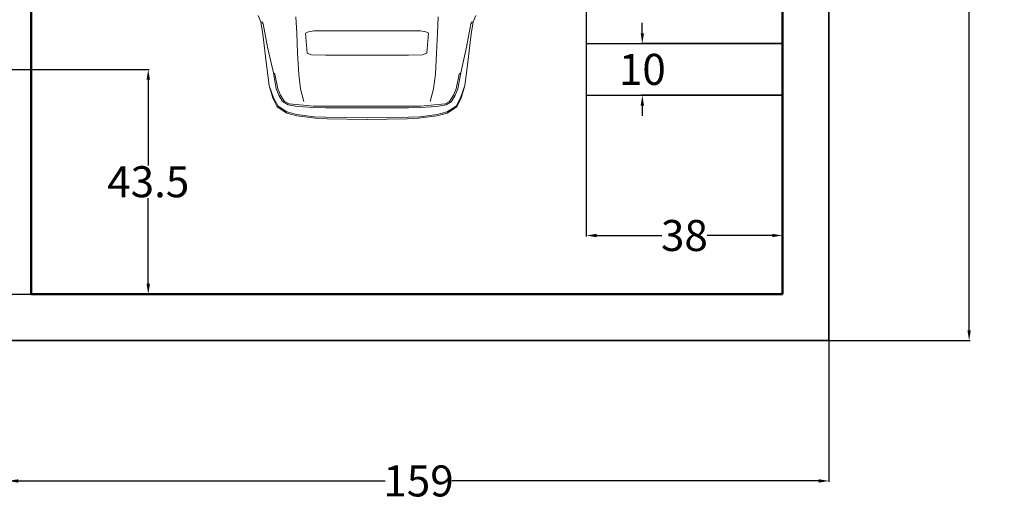
# Model space of a CAD drawing. Units: inches. Extents: x -20 to 10156, y 488 to 2970.
# Tile 2 of 6: x 221 to 412, y 488 to 581. Entities that reach past the tile are written whole.
import ezdxf

# ---------------------------------------------------------------- set-up
doc = ezdxf.new("R2010")
doc.units = ezdxf.units.IN
doc.header["$MEASUREMENT"] = 0
for name, color, linetype, lineweight in [('A-ANNO-DIMS', 2, 'Continuous', 18), ('A-FLOR-STRS', 7, 'Continuous', 25), ('A-FURN-VEHC', 8, 'Continuous', 13), ('A-WALL', 7, 'Continuous', 50), ('C-PROP', 7, 'Continuous', 35)]:
    doc.layers.add(name, color=color, linetype=linetype, lineweight=lineweight)
doc.styles.get("Standard").update_dxf_attribs({"font": 'arial.ttf'})
doc.dimstyles.get("Standard").update_dxf_attribs({"dimtxt": 6, "dimasz": 2, "dimexe": 0.18, "dimexo": 0.0625, "dimgap": 0.09, "dimtad": 0, "dimtih": 1, "dimtoh": 1, "dimdec": 0, "dimzin": 0, "dimdsep": 46, "dimlunit": 4, "dimtxsty": 'Standard', "dimcen": 0.09, "dimadec": 0, "dimazin": 0, "dimtfac": 1, "dimtdec": 0, "dimtofl": 0, "dimtmove": 0, "dimatfit": 3, "dimfxl": 1, "dimtolj": 1, "dimtzin": 0, "dimarcsym": 0})

# ---------------------------------------------------------------- blocks, each defined once
blk = doc.blocks.new('*D14')
at = {"layer": 'A-ANNO-DIMS', "color": 0, "lineweight": -2, "transparency": 16777216}
for p, q in [((206, 618.67), (211.91, 618.67)), ((211.73, 616.67), (211.73, 602.56)), ((211.73, 582.06), (211.73, 596.17)), ((206, 580.06), (211.91, 580.06))]:
    blk.add_line(p, q, dxfattribs=at)
at = {"layer": 'A-ANNO-DIMS', "color": 0, "transparency": 16777216}
for points in [[(211.4, 616.67), (212.07, 616.67), (211.73, 618.67)], [(211.4, 582.06), (212.07, 582.06), (211.73, 580.06)]]:
    blk.add_solid(points, dxfattribs=at)
at = {"layer": 'Defpoints', "color": 0, "transparency": 16777216}
for p in [(205.94, 618.67), (205.94, 580.06), (211.73, 580.06)]:
    blk.add_point(p, dxfattribs=at)
at = {"layer": 'A-ANNO-DIMS', "color": 0, "transparency": 16777216, "insert": (211.73, 599.36), "char_height": 6, "attachment_point": 5}
blk.add_mtext('\\A1;WC 39 TYP.', dxfattribs=at)
blk = doc.blocks.new('*D29')
at = {"layer": 'A-ANNO-DIMS', "color": 0, "lineweight": -2, "transparency": 16777216}
for p, q in [((377.86, 1058.73), (405.13, 1058.73)), ((404.95, 1056.73), (404.95, 791.88)), ((404.95, 520.73), (404.95, 785.58)), ((377.86, 518.73), (405.13, 518.73))]:
    blk.add_line(p, q, dxfattribs=at)
at = {"layer": 'A-ANNO-DIMS', "color": 0, "transparency": 16777216}
for points in [[(404.62, 1056.73), (405.28, 1056.73), (404.95, 1058.73)], [(404.62, 520.73), (405.28, 520.73), (404.95, 518.73)]]:
    blk.add_solid(points, dxfattribs=at)
at = {"layer": 'Defpoints', "color": 0, "transparency": 16777216}
for p in [(377.8, 1058.73), (404.95, 1058.73), (377.8, 518.73)]:
    blk.add_point(p, dxfattribs=at)
at = {"layer": 'A-ANNO-DIMS', "color": 0, "transparency": 16777216, "insert": (404.95, 788.73), "char_height": 6, "attachment_point": 5}
blk.add_mtext('\\A1;540', dxfattribs=at)
blk = doc.blocks.new('*D39')
at = {"layer": 'A-ANNO-DIMS', "color": 0, "lineweight": -2, "transparency": 16777216}
for p, q in [((218.8, 527.67), (218.8, 491.4)), ((377.8, 518.67), (377.8, 491.4)), ((220.8, 491.58), (291.86, 491.58)), ((375.8, 491.58), (304.74, 491.58))]:
    blk.add_line(p, q, dxfattribs=at)
at = {"layer": 'A-ANNO-DIMS', "color": 0, "transparency": 16777216}
for points in [[(220.8, 491.91), (220.8, 491.25), (218.8, 491.58)], [(375.8, 491.91), (375.8, 491.25), (377.8, 491.58)]]:
    blk.add_solid(points, dxfattribs=at)
at = {"layer": 'Defpoints', "color": 0, "transparency": 16777216}
for p in [(218.8, 527.73), (377.8, 518.73), (377.8, 491.58)]:
    blk.add_point(p, dxfattribs=at)
at = {"layer": 'A-ANNO-DIMS', "color": 0, "transparency": 16777216, "insert": (298.3, 491.58), "char_height": 6, "attachment_point": 5}
blk.add_mtext('\\A1;159', dxfattribs=at)
blk = doc.blocks.new('*D40')
at = {"layer": 'A-ANNO-DIMS', "color": 0, "lineweight": -2, "transparency": 16777216}
for p, q in [((218.86, 571.23), (246.13, 571.23)), ((245.95, 569.23), (245.95, 552.64)), ((245.95, 529.73), (245.95, 546.32)), ((218.86, 527.73), (246.13, 527.73))]:
    blk.add_line(p, q, dxfattribs=at)
at = {"layer": 'A-ANNO-DIMS', "color": 0, "transparency": 16777216}
for points in [[(245.62, 569.23), (246.28, 569.23), (245.95, 571.23)], [(245.62, 529.73), (246.28, 529.73), (245.95, 527.73)]]:
    blk.add_solid(points, dxfattribs=at)
at = {"layer": 'Defpoints', "color": 0, "transparency": 16777216}
for p in [(218.8, 571.23), (218.8, 527.73), (245.95, 527.73)]:
    blk.add_point(p, dxfattribs=at)
at = {"layer": 'A-ANNO-DIMS', "color": 0, "transparency": 16777216, "insert": (245.95, 549.48), "char_height": 6, "attachment_point": 5}
blk.add_mtext('\\A1;43.5', dxfattribs=at)
blk = doc.blocks.new('*D41')
at = {"layer": 'A-ANNO-DIMS', "color": 0, "lineweight": -2, "transparency": 16777216}
for p, q in [((330.8, 566.17), (330.8, 538.9)), ((368.8, 566.17), (368.8, 538.9)), ((332.8, 539.08), (345.41, 539.08)), ((366.8, 539.08), (354.19, 539.08))]:
    blk.add_line(p, q, dxfattribs=at)
at = {"layer": 'A-ANNO-DIMS', "color": 0, "transparency": 16777216}
for points in [[(332.8, 539.41), (332.8, 538.75), (330.8, 539.08)], [(366.8, 539.41), (366.8, 538.75), (368.8, 539.08)]]:
    blk.add_solid(points, dxfattribs=at)
at = {"layer": 'Defpoints', "color": 0, "transparency": 16777216}
for p in [(330.8, 566.23), (368.8, 566.23), (330.8, 539.08)]:
    blk.add_point(p, dxfattribs=at)
at = {"layer": 'A-ANNO-DIMS', "color": 0, "transparency": 16777216, "insert": (349.8, 539.08), "char_height": 6, "attachment_point": 5}
blk.add_mtext('\\A1;38', dxfattribs=at)
blk = doc.blocks.new('*D42')
at = {"layer": 'A-ANNO-DIMS', "color": 0, "lineweight": -2, "transparency": 16777216}
for p, q in [((341.65, 578.23), (341.65, 580.23)), ((368.74, 576.23), (341.47, 576.23)), ((368.74, 566.23), (341.47, 566.23)), ((341.65, 564.23), (341.65, 562.23))]:
    blk.add_line(p, q, dxfattribs=at)
at = {"layer": 'A-ANNO-DIMS', "color": 0, "transparency": 16777216}
for points in [[(341.32, 578.23), (341.98, 578.23), (341.65, 576.23)], [(341.32, 564.23), (341.98, 564.23), (341.65, 566.23)]]:
    blk.add_solid(points, dxfattribs=at)
at = {"layer": 'Defpoints', "color": 0, "transparency": 16777216}
for p in [(341.65, 576.23), (368.8, 576.23), (368.8, 566.23)]:
    blk.add_point(p, dxfattribs=at)
at = {"layer": 'A-ANNO-DIMS', "color": 0, "transparency": 16777216, "insert": (341.65, 571.23), "char_height": 6, "attachment_point": 5}
blk.add_mtext('\\A1;10', dxfattribs=at)

msp = doc.modelspace()

# ---------------------------------------------------------------- linework, layer by layer
at = {"layer": 'A-FLOR-STRS'}
for p, q in [((330.8, 676.23), (330.8, 566.23)), ((330.8, 576.23), (368.8, 576.23)), ((330.8, 566.23), (368.8, 566.23))]:
    msp.add_line(p, q, dxfattribs=at)
at = {"layer": 'A-FURN-VEHC'}
for p, q in [((267.26, 581.66, -279.43), (267.75, 580.46, -279.43)), ((267.75, 580.46, -279.43), (268.17, 578.07, -279.43)), ((267.98, 580.46, -279.43), (268.22, 580.04, -279.43)), ((268.22, 580.04, -279.43), (269.07, 575.55, -279.43)), ((274.56, 581.4, -279.43), (274.7, 578.21, -279.43)), ((302.1, 581.4, -279.43), (301.96, 578.21, -279.43)), ((308.45, 580.04, -279.43), (307.6, 575.55, -279.43)), ((308.68, 580.46, -279.43), (308.45, 580.04, -279.43)), ((308.91, 580.46, -279.43), (308.49, 578.07, -279.43)), ((309.4, 581.66, -279.43), (308.91, 580.46, -279.43)), ((268.17, 578.07, -279.43), (268.87, 572.1, -279.43)), ((274.7, 578.21, -279.43), (274.87, 574.38, -279.43)), ((276.42, 578.23, -279.43), (276.97, 578.48, -279.43)), ((276.76, 574.37, -279.43), (276.42, 578.23, -279.43)), ((276.97, 578.48, -279.43), (278.01, 578.66, -279.43)), ((278.01, 578.66, -279.43), (282.63, 578.68, -279.43)), ((282.63, 578.68, -279.43), (288.33, 578.68, -279.43)), ((294.04, 578.68, -279.43), (288.33, 578.68, -279.43)), ((298.66, 578.66, -279.43), (294.04, 578.68, -279.43)), ((299.69, 578.48, -279.43), (298.66, 578.66, -279.43)), ((300.24, 578.23, -279.43), (299.69, 578.48, -279.43)), ((299.9, 574.37, -279.43), (300.24, 578.23, -279.43)), ((301.96, 578.21, -279.43), (301.79, 574.38, -279.43)), ((308.49, 578.07, -279.43), (307.79, 572.1, -279.43)), ((269.07, 575.55, -279.43), (270.19, 570.57, -279.43)), ((274.87, 574.38, -279.43), (275.11, 570.31, -279.43)), ((277.59, 574.05, -279.43), (276.76, 574.37, -279.43)), ((299.08, 574.05, -279.43), (299.9, 574.37, -279.43)), ((301.79, 574.38, -279.43), (301.56, 570.31, -279.43)), ((307.6, 575.55, -279.43), (306.47, 570.57, -279.43)), ((280.32, 573.95, -279.43), (277.59, 574.05, -279.43)), ((288.33, 573.95, -279.43), (280.32, 573.95, -279.43)), ((288.33, 573.95, -279.43), (296.34, 573.95, -279.43)), ((296.34, 573.95, -279.43), (299.08, 574.05, -279.43)), ((268.87, 572.1, -279.43), (269.4, 568.1, -279.43)), ((270.19, 570.57, -279.43), (270.49, 570.31, -279.43)), ((270.19, 570.57, -279.43), (270.72, 567.49, -279.43)), ((270.49, 570.31, -279.43), (271.07, 567.49, -279.43)), ((275.11, 570.31, -279.43), (275.47, 567.49, -279.43)), ((301.56, 570.31, -279.43), (301.19, 567.49, -279.43)), ((306.18, 570.31, -279.43), (305.59, 567.49, -279.43)), ((306.47, 570.57, -279.43), (305.94, 567.49, -279.43)), ((306.47, 570.57, -279.43), (306.18, 570.31, -279.43)), ((307.79, 572.1, -279.43), (307.26, 568.1, -279.43)), ((270.07, 565.66, -279.43), (269.4, 568.1, -279.43)), ((269.4, 568.1, -279.43), (270.23, 565.71, -279.43)), ((270.72, 567.49, -279.43), (271.24, 566.22, -279.43)), ((271.07, 567.49, -279.43), (271.59, 566.22, -279.43)), ((275.47, 567.49, -279.43), (275.76, 566.22, -279.43)), ((301.19, 567.49, -279.43), (300.9, 566.22, -279.43)), ((305.59, 567.49, -279.43), (305.07, 566.22, -279.43)), ((305.94, 567.49, -279.43), (305.42, 566.22, -279.43)), ((307.26, 568.1, -279.43), (306.43, 565.71, -279.43)), ((306.59, 565.66, -279.43), (307.26, 568.1, -279.43)), ((270.93, 564, -279.43), (270.07, 565.66, -279.43)), ((270.23, 565.71, -279.43), (271.09, 564.11, -279.43)), ((271.24, 566.22, -279.43), (271.96, 565.03, -279.43)), ((271.59, 566.22, -279.43), (272.36, 565.03, -279.43)), ((271.96, 565.03, -279.43), (273.02, 564.38, -279.43)), ((272.36, 565.03, -279.43), (273.23, 564.59, -279.43)), ((273.23, 564.59, -279.43), (277.98, 564.11, -279.43)), ((275.76, 566.22, -279.43), (276.11, 565.03, -279.43)), ((303.43, 564.59, -279.43), (298.68, 564.11, -279.43)), ((300.9, 566.22, -279.43), (300.55, 565.03, -279.43)), ((304.3, 565.03, -279.43), (303.43, 564.59, -279.43)), ((304.7, 565.03, -279.43), (303.64, 564.38, -279.43)), ((305.07, 566.22, -279.43), (304.3, 565.03, -279.43)), ((305.42, 566.22, -279.43), (304.7, 565.03, -279.43)), ((306.43, 565.71, -279.43), (305.57, 564.11, -279.43)), ((305.73, 564, -279.43), (306.59, 565.66, -279.43)), ((272.81, 562.76, -279.43), (270.93, 564, -279.43)), ((271.09, 564.11, -279.43), (272.81, 563.01, -279.43)), ((272.81, 563.01, -279.43), (274.75, 562.48, -279.43)), ((274.75, 562.22, -279.43), (272.81, 562.76, -279.43)), ((273.02, 564.38, -279.43), (274.83, 564.06, -279.43)), ((274.83, 564.06, -279.43), (278.02, 563.85, -279.43)), ((277.98, 564.11, -279.43), (280.29, 564.08, -279.43)), ((278.02, 563.85, -279.43), (280.31, 563.77, -279.43)), ((296.37, 564.08, -279.43), (280.29, 564.08, -279.43)), ((280.31, 563.77, -279.43), (296.35, 563.77, -279.43)), ((298.65, 563.85, -279.43), (296.35, 563.77, -279.43)), ((298.68, 564.11, -279.43), (296.37, 564.08, -279.43)), ((301.83, 564.06, -279.43), (298.65, 563.85, -279.43)), ((303.64, 564.38, -279.43), (301.83, 564.06, -279.43)), ((303.85, 563.01, -279.43), (301.92, 562.48, -279.43)), ((301.92, 562.22, -279.43), (303.85, 562.76, -279.43)), ((305.57, 564.11, -279.43), (303.85, 563.01, -279.43)), ((303.85, 562.76, -279.43), (305.73, 564, -279.43)), ((274.75, 562.48, -279.43), (278.11, 562.06, -279.43)), ((278.37, 561.78, -279.43), (274.75, 562.22, -279.43)), ((278.11, 562.06, -279.43), (280.33, 561.96, -279.43)), ((280.59, 561.68, -279.43), (278.37, 561.78, -279.43)), ((280.33, 561.96, -279.43), (288.33, 561.87, -279.43)), ((288.32, 561.53, -279.43), (280.59, 561.68, -279.43)), ((296.33, 561.96, -279.43), (288.33, 561.87, -279.43)), ((288.34, 561.53, -279.43), (296.07, 561.68, -279.43)), ((296.07, 561.68, -279.43), (298.3, 561.78, -279.43)), ((298.55, 562.06, -279.43), (296.33, 561.96, -279.43)), ((298.3, 561.78, -279.43), (301.92, 562.22, -279.43)), ((301.92, 562.48, -279.43), (298.55, 562.06, -279.43))]:
    msp.add_line(p, q, dxfattribs=at)
at = {"layer": 'A-WALL'}
for p, q in [((223.3, 527.73), (223.3, 724.23)), ((368.8, 724.23), (368.8, 527.73)), ((368.8, 527.73), (223.3, 527.73))]:
    msp.add_line(p, q, dxfattribs=at)
at = {"layer": 'C-PROP'}
for p, q in [((377.8, 1058.73), (377.8, 518.73)), ((377.8, 518.73), (17.8, 518.73))]:
    msp.add_line(p, q, dxfattribs=at)

# ---------------------------------------------------------------- dimensions: what is measured, and where the dimension line sits
at = {"layer": 'A-ANNO-DIMS'}
for base, p1, p2, angle, override, picture, middle in [((404.95, 1058.73), (377.8, 518.73), (377.8, 1058.73), 90, {"dimdec": 0, "dimlfac": 1, "dimrnd": 0, "dimzin": 0, "dimdsep": 46, "dimlunit": 2}, '*D29', (404.95, 788.73)), ((341.65, 576.23), (368.8, 566.23), (368.8, 576.23), 90, {"dimdec": 0, "dimlfac": 1, "dimrnd": 0, "dimzin": 0, "dimdsep": 46, "dimlunit": 2}, '*D42', (341.65, 571.23)), ((245.95, 527.73), (218.8, 571.23), (218.8, 527.73), 270, {"dimdec": 1, "dimlfac": 1, "dimrnd": 0, "dimzin": 0, "dimdsep": 46, "dimlunit": 2}, '*D40', (245.95, 549.48)), ((330.8, 539.08), (368.8, 566.23), (330.8, 566.23), 180, {"dimdec": 0, "dimlfac": 1, "dimrnd": 0, "dimzin": 0, "dimdsep": 46, "dimlunit": 2}, '*D41', (349.8, 539.08))]:
    dim = msp.add_linear_dim(base=base, p1=p1, p2=p2, angle=angle, dimstyle='Standard', override=override, dxfattribs=at)
    dim.commit()
    dim.dimension.update_dxf_attribs({"geometry": picture, "text_midpoint": middle})
dim = msp.add_linear_dim(base=(211.73, 580.06), p1=(205.94, 618.67), p2=(205.94, 580.06), angle=270, text='WC <> TYP.', dimstyle='Standard', override={"dimdec": 0, "dimlfac": 1, "dimrnd": 0, "dimzin": 0, "dimdsep": 46, "dimlunit": 2}, dxfattribs=at)
dim.commit()
dim.dimension.update_dxf_attribs({"geometry": '*D14', "text_midpoint": (211.73, 599.36)})
dim = msp.add_linear_dim(base=(377.8, 491.58), p1=(218.8, 527.73), p2=(377.8, 518.73), dimstyle='Standard', override={"dimdec": 0, "dimlfac": 1, "dimrnd": 0, "dimzin": 0, "dimdsep": 46, "dimlunit": 2}, dxfattribs=at)
dim.commit()
dim.dimension.update_dxf_attribs({"geometry": '*D39', "text_midpoint": (298.3, 491.58)})

doc.saveas('drawing.dxf')
